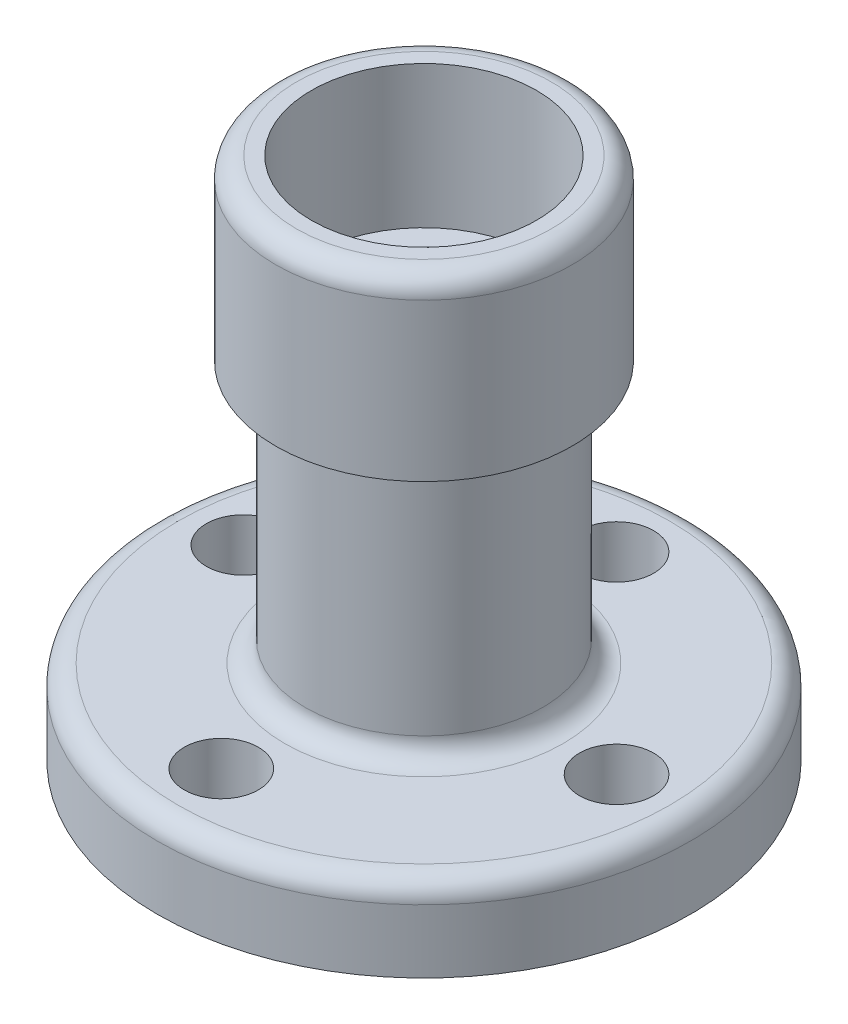
ISO-10303-21;
HEADER;
FILE_DESCRIPTION(('STEP AP214'),'2;1');
FILE_NAME('part.step','',(''),(''),'','','');
FILE_SCHEMA(('AUTOMOTIVE_DESIGN { 1 0 10303 214 1 1 1 1 }'));
ENDSEC;
DATA;
#1=APPLICATION_CONTEXT('core data for automotive mechanical design processes');
#2=APPLICATION_PROTOCOL_DEFINITION('international standard','automotive_design',2000,#1);
#3=PRODUCT_CONTEXT('',#1,'mechanical');
#4=PRODUCT('Part','Part','',(#3));
#5=PRODUCT_RELATED_PRODUCT_CATEGORY('part','',(#4));
#6=PRODUCT_DEFINITION_FORMATION('','',#4);
#7=PRODUCT_DEFINITION_CONTEXT('part definition',#1,'design');
#8=PRODUCT_DEFINITION('design','',#6,#7);
#9=PRODUCT_DEFINITION_SHAPE('','',#8);
#10=(LENGTH_UNIT() NAMED_UNIT(*) SI_UNIT(.MILLI.,.METRE.));
#11=(NAMED_UNIT(*) PLANE_ANGLE_UNIT() SI_UNIT($,.RADIAN.));
#12=(NAMED_UNIT(*) SI_UNIT($,.STERADIAN.) SOLID_ANGLE_UNIT());
#13=UNCERTAINTY_MEASURE_WITH_UNIT(LENGTH_MEASURE(1.E-05),#10,'distance_accuracy_value','');
#14=(GEOMETRIC_REPRESENTATION_CONTEXT(3) GLOBAL_UNCERTAINTY_ASSIGNED_CONTEXT((#13)) GLOBAL_UNIT_ASSIGNED_CONTEXT((#10,
#11,#12)) REPRESENTATION_CONTEXT('',''));
#15=CARTESIAN_POINT('',(0.,0.,0.));
#16=DIRECTION('',(0.,0.,1.));
#17=DIRECTION('',(1.,0.,0.));
#18=AXIS2_PLACEMENT_3D('',#15,#16,#17);
#19=CARTESIAN_POINT('',(0.,14.2,0.));
#20=DIRECTION('',(0.,-1.,0.));
#21=DIRECTION('',(0.,0.,-1.));
#22=AXIS2_PLACEMENT_3D('',#19,#20,#21);
#23=CYLINDRICAL_SURFACE('',#22,45.);
#24=CARTESIAN_POINT('',(0.,10.7,0.));
#25=DIRECTION('',(0.,1.,0.));
#26=DIRECTION('',(0.,0.,1.));
#27=AXIS2_PLACEMENT_3D('',#24,#25,#26);
#28=CIRCLE('',#27,45.);
#29=CARTESIAN_POINT('',(0.,10.7,45.));
#30=VERTEX_POINT('',#29);
#31=EDGE_CURVE('E10',#30,#30,#28,.F.);
#32=ORIENTED_EDGE('',*,*,#31,.T.);
#33=EDGE_LOOP('',(#32));
#34=FACE_BOUND('',#33,.T.);
#35=CARTESIAN_POINT('',(0.,0.,0.));
#36=DIRECTION('',(0.,1.,0.));
#37=DIRECTION('',(0.,0.,1.));
#38=AXIS2_PLACEMENT_3D('',#35,#36,#37);
#39=CIRCLE('',#38,45.);
#40=CARTESIAN_POINT('',(0.,0.,45.));
#41=VERTEX_POINT('',#40);
#42=EDGE_CURVE('E66',#41,#41,#39,.T.);
#43=ORIENTED_EDGE('',*,*,#42,.T.);
#44=EDGE_LOOP('',(#43));
#45=FACE_BOUND('',#44,.T.);
#46=ADVANCED_FACE('F40',(#34,#45),#23,.T.);
#47=CARTESIAN_POINT('',(0.,14.2,0.));
#48=DIRECTION('',(0.,1.,0.));
#49=DIRECTION('',(0.,0.,1.));
#50=AXIS2_PLACEMENT_3D('',#47,#48,#49);
#51=PLANE('',#50);
#52=CARTESIAN_POINT('',(0.,14.2,0.));
#53=DIRECTION('',(0.,1.,0.));
#54=DIRECTION('',(0.,0.,1.));
#55=AXIS2_PLACEMENT_3D('',#52,#53,#54);
#56=CIRCLE('',#55,41.5);
#57=CARTESIAN_POINT('',(0.,14.2,41.5));
#58=VERTEX_POINT('',#57);
#59=EDGE_CURVE('E42',#58,#58,#56,.T.);
#60=ORIENTED_EDGE('',*,*,#59,.T.);
#61=EDGE_LOOP('',(#60));
#62=FACE_BOUND('',#61,.T.);
#63=CARTESIAN_POINT('',(0.,14.2,0.));
#64=DIRECTION('',(0.,1.,0.));
#65=DIRECTION('',(0.,0.,1.));
#66=AXIS2_PLACEMENT_3D('',#63,#64,#65);
#67=CIRCLE('',#66,23.5);
#68=CARTESIAN_POINT('',(0.,14.2,23.5));
#69=VERTEX_POINT('',#68);
#70=EDGE_CURVE('E62',#69,#69,#67,.F.);
#71=ORIENTED_EDGE('',*,*,#70,.T.);
#72=EDGE_LOOP('',(#71));
#73=FACE_BOUND('',#72,.T.);
#74=CARTESIAN_POINT('',(-1.69244395993731,14.2,32.5));
#75=DIRECTION('',(0.,1.,0.));
#76=DIRECTION('',(0.,0.,1.));
#77=AXIS2_PLACEMENT_3D('',#74,#75,#76);
#78=CIRCLE('',#77,6.25);
#79=CARTESIAN_POINT('',(-1.69244395993731,14.2,38.75));
#80=VERTEX_POINT('',#79);
#81=EDGE_CURVE('E76',#80,#80,#78,.T.);
#82=ORIENTED_EDGE('',*,*,#81,.F.);
#83=EDGE_LOOP('',(#82));
#84=FACE_BOUND('',#83,.T.);
#85=CARTESIAN_POINT('',(-32.5,14.2,-2.03093275192457));
#86=DIRECTION('',(0.,1.,0.));
#87=DIRECTION('',(0.,0.,1.));
#88=AXIS2_PLACEMENT_3D('',#85,#86,#87);
#89=CIRCLE('',#88,6.25);
#90=CARTESIAN_POINT('',(-32.5,14.2,4.21906724807543));
#91=VERTEX_POINT('',#90);
#92=EDGE_CURVE('E80',#91,#91,#89,.T.);
#93=ORIENTED_EDGE('',*,*,#92,.F.);
#94=EDGE_LOOP('',(#93));
#95=FACE_BOUND('',#94,.T.);
#96=CARTESIAN_POINT('',(32.5,14.2,0.));
#97=DIRECTION('',(0.,1.,0.));
#98=DIRECTION('',(0.,0.,1.));
#99=AXIS2_PLACEMENT_3D('',#96,#97,#98);
#100=CIRCLE('',#99,6.25);
#101=CARTESIAN_POINT('',(32.5,14.2,6.25));
#102=VERTEX_POINT('',#101);
#103=EDGE_CURVE('E84',#102,#102,#100,.T.);
#104=ORIENTED_EDGE('',*,*,#103,.F.);
#105=EDGE_LOOP('',(#104));
#106=FACE_BOUND('',#105,.T.);
#107=CARTESIAN_POINT('',(0.,14.2,-32.5));
#108=DIRECTION('',(0.,1.,0.));
#109=DIRECTION('',(0.,0.,1.));
#110=AXIS2_PLACEMENT_3D('',#107,#108,#109);
#111=CIRCLE('',#110,6.25);
#112=CARTESIAN_POINT('',(0.,14.2,-26.25));
#113=VERTEX_POINT('',#112);
#114=EDGE_CURVE('E87',#113,#113,#111,.T.);
#115=ORIENTED_EDGE('',*,*,#114,.F.);
#116=EDGE_LOOP('',(#115));
#117=FACE_BOUND('',#116,.T.);
#118=ADVANCED_FACE('F121',(#62,#73,#84,#95,#106,#117),#51,.T.);
#119=CARTESIAN_POINT('',(0.,0.,0.));
#120=DIRECTION('',(0.,1.,0.));
#121=DIRECTION('',(0.,0.,1.));
#122=AXIS2_PLACEMENT_3D('',#119,#120,#121);
#123=PLANE('',#122);
#124=CARTESIAN_POINT('',(0.,0.,0.));
#125=DIRECTION('',(0.,-1.,0.));
#126=DIRECTION('',(0.,0.,-1.));
#127=AXIS2_PLACEMENT_3D('',#124,#125,#126);
#128=CIRCLE('',#127,15.);
#129=CARTESIAN_POINT('',(0.,0.,-15.));
#130=VERTEX_POINT('',#129);
#131=EDGE_CURVE('E73',#130,#130,#128,.T.);
#132=ORIENTED_EDGE('',*,*,#131,.F.);
#133=EDGE_LOOP('',(#132));
#134=FACE_BOUND('',#133,.T.);
#135=CARTESIAN_POINT('',(-1.69244395993731,0.,32.5));
#136=DIRECTION('',(0.,1.,0.));
#137=DIRECTION('',(0.,0.,1.));
#138=AXIS2_PLACEMENT_3D('',#135,#136,#137);
#139=CIRCLE('',#138,6.25);
#140=CARTESIAN_POINT('',(-1.69244395993731,0.,38.75));
#141=VERTEX_POINT('',#140);
#142=EDGE_CURVE('E74',#141,#141,#139,.T.);
#143=ORIENTED_EDGE('',*,*,#142,.T.);
#144=EDGE_LOOP('',(#143));
#145=FACE_BOUND('',#144,.T.);
#146=CARTESIAN_POINT('',(-32.5,0.,-2.03093275192457));
#147=DIRECTION('',(0.,1.,0.));
#148=DIRECTION('',(0.,0.,1.));
#149=AXIS2_PLACEMENT_3D('',#146,#147,#148);
#150=CIRCLE('',#149,6.25);
#151=CARTESIAN_POINT('',(-32.5,0.,4.21906724807543));
#152=VERTEX_POINT('',#151);
#153=EDGE_CURVE('E79',#152,#152,#150,.T.);
#154=ORIENTED_EDGE('',*,*,#153,.T.);
#155=EDGE_LOOP('',(#154));
#156=FACE_BOUND('',#155,.T.);
#157=CARTESIAN_POINT('',(32.5,0.,0.));
#158=DIRECTION('',(0.,1.,0.));
#159=DIRECTION('',(0.,0.,1.));
#160=AXIS2_PLACEMENT_3D('',#157,#158,#159);
#161=CIRCLE('',#160,6.25);
#162=CARTESIAN_POINT('',(32.5,0.,6.25));
#163=VERTEX_POINT('',#162);
#164=EDGE_CURVE('E82',#163,#163,#161,.T.);
#165=ORIENTED_EDGE('',*,*,#164,.T.);
#166=EDGE_LOOP('',(#165));
#167=FACE_BOUND('',#166,.T.);
#168=CARTESIAN_POINT('',(0.,0.,-32.5));
#169=DIRECTION('',(0.,1.,0.));
#170=DIRECTION('',(0.,0.,1.));
#171=AXIS2_PLACEMENT_3D('',#168,#169,#170);
#172=CIRCLE('',#171,6.25);
#173=CARTESIAN_POINT('',(0.,0.,-26.25));
#174=VERTEX_POINT('',#173);
#175=EDGE_CURVE('E90',#174,#174,#172,.T.);
#176=ORIENTED_EDGE('',*,*,#175,.T.);
#177=EDGE_LOOP('',(#176));
#178=FACE_BOUND('',#177,.T.);
#179=ORIENTED_EDGE('',*,*,#42,.F.);
#180=EDGE_LOOP('',(#179));
#181=FACE_BOUND('',#180,.T.);
#182=ADVANCED_FACE('F119',(#134,#145,#156,#167,#178,#181),#123,.F.);
#183=CARTESIAN_POINT('',(0.,58.4,0.));
#184=DIRECTION('',(0.,-1.,0.));
#185=DIRECTION('',(0.,0.,-1.));
#186=AXIS2_PLACEMENT_3D('',#183,#184,#185);
#187=CYLINDRICAL_SURFACE('',#186,20.);
#188=CARTESIAN_POINT('',(0.,54.9,0.));
#189=DIRECTION('',(0.,1.,0.));
#190=DIRECTION('',(0.,0.,1.));
#191=AXIS2_PLACEMENT_3D('',#188,#189,#190);
#192=CIRCLE('',#191,20.);
#193=CARTESIAN_POINT('',(0.,54.9,20.));
#194=VERTEX_POINT('',#193);
#195=EDGE_CURVE('E48',#194,#194,#192,.F.);
#196=ORIENTED_EDGE('',*,*,#195,.T.);
#197=EDGE_LOOP('',(#196));
#198=FACE_BOUND('',#197,.T.);
#199=CARTESIAN_POINT('',(0.,17.7,0.));
#200=DIRECTION('',(0.,1.,0.));
#201=DIRECTION('',(0.,0.,1.));
#202=AXIS2_PLACEMENT_3D('',#199,#200,#201);
#203=CIRCLE('',#202,20.);
#204=CARTESIAN_POINT('',(0.,17.7,20.));
#205=VERTEX_POINT('',#204);
#206=EDGE_CURVE('E67',#205,#205,#203,.T.);
#207=ORIENTED_EDGE('',*,*,#206,.T.);
#208=EDGE_LOOP('',(#207));
#209=FACE_BOUND('',#208,.T.);
#210=ADVANCED_FACE('F124',(#198,#209),#187,.T.);
#211=CARTESIAN_POINT('',(0.,88.4,0.));
#212=DIRECTION('',(0.,-1.,0.));
#213=DIRECTION('',(0.,0.,-1.));
#214=AXIS2_PLACEMENT_3D('',#211,#212,#213);
#215=CYLINDRICAL_SURFACE('',#214,25.);
#216=CARTESIAN_POINT('',(0.,84.9,0.));
#217=DIRECTION('',(0.,1.,0.));
#218=DIRECTION('',(0.,0.,1.));
#219=AXIS2_PLACEMENT_3D('',#216,#217,#218);
#220=CIRCLE('',#219,25.);
#221=CARTESIAN_POINT('',(0.,84.9,25.));
#222=VERTEX_POINT('',#221);
#223=EDGE_CURVE('E60',#222,#222,#220,.F.);
#224=ORIENTED_EDGE('',*,*,#223,.T.);
#225=EDGE_LOOP('',(#224));
#226=FACE_BOUND('',#225,.T.);
#227=CARTESIAN_POINT('',(0.,58.4,0.));
#228=DIRECTION('',(0.,1.,0.));
#229=DIRECTION('',(0.,0.,1.));
#230=AXIS2_PLACEMENT_3D('',#227,#228,#229);
#231=CIRCLE('',#230,25.);
#232=CARTESIAN_POINT('',(0.,58.4,25.));
#233=VERTEX_POINT('',#232);
#234=EDGE_CURVE('E88',#233,#233,#231,.T.);
#235=ORIENTED_EDGE('',*,*,#234,.T.);
#236=EDGE_LOOP('',(#235));
#237=FACE_BOUND('',#236,.T.);
#238=ADVANCED_FACE('F167',(#226,#237),#215,.T.);
#239=CARTESIAN_POINT('',(0.,88.4,0.));
#240=DIRECTION('',(0.,1.,0.));
#241=DIRECTION('',(0.,0.,1.));
#242=AXIS2_PLACEMENT_3D('',#239,#240,#241);
#243=PLANE('',#242);
#244=CARTESIAN_POINT('',(0.,88.4,0.));
#245=DIRECTION('',(0.,1.,0.));
#246=DIRECTION('',(0.,0.,1.));
#247=AXIS2_PLACEMENT_3D('',#244,#245,#246);
#248=CIRCLE('',#247,21.5);
#249=CARTESIAN_POINT('',(0.,88.4,21.5));
#250=VERTEX_POINT('',#249);
#251=EDGE_CURVE('E58',#250,#250,#248,.T.);
#252=ORIENTED_EDGE('',*,*,#251,.T.);
#253=EDGE_LOOP('',(#252));
#254=FACE_BOUND('',#253,.T.);
#255=CARTESIAN_POINT('',(0.,88.4,0.));
#256=DIRECTION('',(0.,1.,0.));
#257=DIRECTION('',(0.,0.,1.));
#258=AXIS2_PLACEMENT_3D('',#255,#256,#257);
#259=CIRCLE('',#258,19.);
#260=CARTESIAN_POINT('',(0.,88.4,19.));
#261=VERTEX_POINT('',#260);
#262=EDGE_CURVE('E101',#261,#261,#259,.T.);
#263=ORIENTED_EDGE('',*,*,#262,.F.);
#264=EDGE_LOOP('',(#263));
#265=FACE_BOUND('',#264,.T.);
#266=ADVANCED_FACE('F168',(#254,#265),#243,.T.);
#267=CARTESIAN_POINT('',(0.,58.4,0.));
#268=DIRECTION('',(0.,1.,0.));
#269=DIRECTION('',(0.,0.,1.));
#270=AXIS2_PLACEMENT_3D('',#267,#268,#269);
#271=PLANE('',#270);
#272=CARTESIAN_POINT('',(0.,58.4,0.));
#273=DIRECTION('',(0.,1.,0.));
#274=DIRECTION('',(0.,0.,1.));
#275=AXIS2_PLACEMENT_3D('',#272,#273,#274);
#276=CIRCLE('',#275,23.5);
#277=CARTESIAN_POINT('',(0.,58.4,23.5));
#278=VERTEX_POINT('',#277);
#279=EDGE_CURVE('E55',#278,#278,#276,.T.);
#280=ORIENTED_EDGE('',*,*,#279,.T.);
#281=EDGE_LOOP('',(#280));
#282=FACE_BOUND('',#281,.T.);
#283=ORIENTED_EDGE('',*,*,#234,.F.);
#284=EDGE_LOOP('',(#283));
#285=FACE_BOUND('',#284,.T.);
#286=ADVANCED_FACE('F161',(#282,#285),#271,.F.);
#287=CARTESIAN_POINT('',(0.,-15.8,-32.5));
#288=DIRECTION('',(0.,1.,0.));
#289=DIRECTION('',(0.,0.,1.));
#290=AXIS2_PLACEMENT_3D('',#287,#288,#289);
#291=CYLINDRICAL_SURFACE('',#290,6.25);
#292=ORIENTED_EDGE('',*,*,#114,.T.);
#293=EDGE_LOOP('',(#292));
#294=FACE_BOUND('',#293,.T.);
#295=ORIENTED_EDGE('',*,*,#175,.F.);
#296=EDGE_LOOP('',(#295));
#297=FACE_BOUND('',#296,.T.);
#298=ADVANCED_FACE('F164',(#294,#297),#291,.F.);
#299=CARTESIAN_POINT('',(32.5,-15.8,0.));
#300=DIRECTION('',(0.,1.,0.));
#301=DIRECTION('',(0.,0.,1.));
#302=AXIS2_PLACEMENT_3D('',#299,#300,#301);
#303=CYLINDRICAL_SURFACE('',#302,6.25);
#304=ORIENTED_EDGE('',*,*,#103,.T.);
#305=EDGE_LOOP('',(#304));
#306=FACE_BOUND('',#305,.T.);
#307=ORIENTED_EDGE('',*,*,#164,.F.);
#308=EDGE_LOOP('',(#307));
#309=FACE_BOUND('',#308,.T.);
#310=ADVANCED_FACE('F184',(#306,#309),#303,.F.);
#311=CARTESIAN_POINT('',(-32.5,-15.8,-2.03093275192457));
#312=DIRECTION('',(0.,1.,0.));
#313=DIRECTION('',(0.,0.,1.));
#314=AXIS2_PLACEMENT_3D('',#311,#312,#313);
#315=CYLINDRICAL_SURFACE('',#314,6.25);
#316=ORIENTED_EDGE('',*,*,#92,.T.);
#317=EDGE_LOOP('',(#316));
#318=FACE_BOUND('',#317,.T.);
#319=ORIENTED_EDGE('',*,*,#153,.F.);
#320=EDGE_LOOP('',(#319));
#321=FACE_BOUND('',#320,.T.);
#322=ADVANCED_FACE('F186',(#318,#321),#315,.F.);
#323=CARTESIAN_POINT('',(-1.69244395993731,-15.8,32.5));
#324=DIRECTION('',(0.,1.,0.));
#325=DIRECTION('',(0.,0.,1.));
#326=AXIS2_PLACEMENT_3D('',#323,#324,#325);
#327=CYLINDRICAL_SURFACE('',#326,6.25);
#328=ORIENTED_EDGE('',*,*,#81,.T.);
#329=EDGE_LOOP('',(#328));
#330=FACE_BOUND('',#329,.T.);
#331=ORIENTED_EDGE('',*,*,#142,.F.);
#332=EDGE_LOOP('',(#331));
#333=FACE_BOUND('',#332,.T.);
#334=ADVANCED_FACE('F192',(#330,#333),#327,.F.);
#335=CARTESIAN_POINT('',(0.,76.4,0.));
#336=DIRECTION('',(0.,1.,0.));
#337=DIRECTION('',(0.,0.,1.));
#338=AXIS2_PLACEMENT_3D('',#335,#336,#337);
#339=CYLINDRICAL_SURFACE('',#338,19.);
#340=ORIENTED_EDGE('',*,*,#262,.T.);
#341=EDGE_LOOP('',(#340));
#342=FACE_BOUND('',#341,.T.);
#343=CARTESIAN_POINT('',(0.,64.4,0.));
#344=DIRECTION('',(0.,1.,0.));
#345=DIRECTION('',(0.,0.,1.));
#346=AXIS2_PLACEMENT_3D('',#343,#344,#345);
#347=CIRCLE('',#346,19.);
#348=CARTESIAN_POINT('',(0.,64.4,19.));
#349=VERTEX_POINT('',#348);
#350=EDGE_CURVE('E106',#349,#349,#347,.T.);
#351=ORIENTED_EDGE('',*,*,#350,.F.);
#352=EDGE_LOOP('',(#351));
#353=FACE_BOUND('',#352,.T.);
#354=ADVANCED_FACE('F200',(#342,#353),#339,.F.);
#355=CARTESIAN_POINT('',(0.,64.4,0.));
#356=DIRECTION('',(0.,1.,0.));
#357=DIRECTION('',(0.,0.,1.));
#358=AXIS2_PLACEMENT_3D('',#355,#356,#357);
#359=PLANE('',#358);
#360=CARTESIAN_POINT('',(0.,64.4,0.));
#361=DIRECTION('',(0.,1.,0.));
#362=DIRECTION('',(0.,0.,1.));
#363=AXIS2_PLACEMENT_3D('',#360,#361,#362);
#364=CIRCLE('',#363,15.);
#365=CARTESIAN_POINT('',(0.,64.4,15.));
#366=VERTEX_POINT('',#365);
#367=EDGE_CURVE('E107',#366,#366,#364,.T.);
#368=ORIENTED_EDGE('',*,*,#367,.F.);
#369=EDGE_LOOP('',(#368));
#370=FACE_BOUND('',#369,.T.);
#371=ORIENTED_EDGE('',*,*,#350,.T.);
#372=EDGE_LOOP('',(#371));
#373=FACE_BOUND('',#372,.T.);
#374=ADVANCED_FACE('F202',(#370,#373),#359,.T.);
#375=CARTESIAN_POINT('',(0.,58.4,0.));
#376=DIRECTION('',(0.,1.,0.));
#377=DIRECTION('',(0.,0.,1.));
#378=AXIS2_PLACEMENT_3D('',#375,#376,#377);
#379=CYLINDRICAL_SURFACE('',#378,15.);
#380=ORIENTED_EDGE('',*,*,#367,.T.);
#381=EDGE_LOOP('',(#380));
#382=FACE_BOUND('',#381,.T.);
#383=CARTESIAN_POINT('',(0.,3.5,0.));
#384=DIRECTION('',(0.,-1.,0.));
#385=DIRECTION('',(0.,0.,-1.));
#386=AXIS2_PLACEMENT_3D('',#383,#384,#385);
#387=CIRCLE('',#386,15.);
#388=CARTESIAN_POINT('',(0.,3.5,-15.));
#389=VERTEX_POINT('',#388);
#390=EDGE_CURVE('E68',#389,#389,#387,.T.);
#391=ORIENTED_EDGE('',*,*,#390,.T.);
#392=EDGE_LOOP('',(#391));
#393=FACE_BOUND('',#392,.T.);
#394=ADVANCED_FACE('F201',(#382,#393),#379,.F.);
#395=CARTESIAN_POINT('',(0.,0.,0.));
#396=DIRECTION('',(0.,1.,0.));
#397=DIRECTION('',(0.,0.,-1.));
#398=AXIS2_PLACEMENT_3D('',#395,#396,#397);
#399=CONICAL_SURFACE('',#398,15.,0.0610865238198017);
#400=CARTESIAN_POINT('',(0.,3.5,0.));
#401=DIRECTION('',(0.,-1.,0.));
#402=DIRECTION('',(0.,0.,-1.));
#403=AXIS2_PLACEMENT_3D('',#400,#401,#402);
#404=CIRCLE('',#403,15.2140691705267);
#405=CARTESIAN_POINT('',(0.,3.5,-15.2140691705267));
#406=VERTEX_POINT('',#405);
#407=EDGE_CURVE('E115',#406,#406,#404,.T.);
#408=ORIENTED_EDGE('',*,*,#407,.F.);
#409=EDGE_LOOP('',(#408));
#410=FACE_BOUND('',#409,.T.);
#411=ORIENTED_EDGE('',*,*,#131,.T.);
#412=EDGE_LOOP('',(#411));
#413=FACE_BOUND('',#412,.T.);
#414=ADVANCED_FACE('F117',(#410,#413),#399,.F.);
#415=CARTESIAN_POINT('',(0.,3.5,0.));
#416=DIRECTION('',(0.,-1.,0.));
#417=DIRECTION('',(0.,0.,-1.));
#418=AXIS2_PLACEMENT_3D('',#415,#416,#417);
#419=PLANE('',#418);
#420=ORIENTED_EDGE('',*,*,#390,.F.);
#421=EDGE_LOOP('',(#420));
#422=FACE_BOUND('',#421,.T.);
#423=ORIENTED_EDGE('',*,*,#407,.T.);
#424=EDGE_LOOP('',(#423));
#425=FACE_BOUND('',#424,.T.);
#426=ADVANCED_FACE('F147',(#422,#425),#419,.T.);
#427=CARTESIAN_POINT('',(0.,17.7,0.));
#428=DIRECTION('',(0.,1.,0.));
#429=DIRECTION('',(0.,0.,1.));
#430=AXIS2_PLACEMENT_3D('',#427,#428,#429);
#431=TOROIDAL_SURFACE('',#430,23.5,3.5);
#432=ORIENTED_EDGE('',*,*,#70,.F.);
#433=EDGE_LOOP('',(#432));
#434=FACE_BOUND('',#433,.T.);
#435=ORIENTED_EDGE('',*,*,#206,.F.);
#436=EDGE_LOOP('',(#435));
#437=FACE_BOUND('',#436,.T.);
#438=ADVANCED_FACE('F144',(#434,#437),#431,.F.);
#439=CARTESIAN_POINT('',(0.,84.9,0.));
#440=DIRECTION('',(0.,1.,0.));
#441=DIRECTION('',(0.,0.,1.));
#442=AXIS2_PLACEMENT_3D('',#439,#440,#441);
#443=TOROIDAL_SURFACE('',#442,21.5,3.5);
#444=ORIENTED_EDGE('',*,*,#223,.F.);
#445=EDGE_LOOP('',(#444));
#446=FACE_BOUND('',#445,.T.);
#447=ORIENTED_EDGE('',*,*,#251,.F.);
#448=EDGE_LOOP('',(#447));
#449=FACE_BOUND('',#448,.T.);
#450=ADVANCED_FACE('F149',(#446,#449),#443,.T.);
#451=CARTESIAN_POINT('',(0.,54.9,0.));
#452=DIRECTION('',(0.,1.,0.));
#453=DIRECTION('',(0.,0.,1.));
#454=AXIS2_PLACEMENT_3D('',#451,#452,#453);
#455=TOROIDAL_SURFACE('',#454,23.5,3.5);
#456=ORIENTED_EDGE('',*,*,#195,.F.);
#457=EDGE_LOOP('',(#456));
#458=FACE_BOUND('',#457,.T.);
#459=ORIENTED_EDGE('',*,*,#279,.F.);
#460=EDGE_LOOP('',(#459));
#461=FACE_BOUND('',#460,.T.);
#462=ADVANCED_FACE('F152',(#458,#461),#455,.F.);
#463=CARTESIAN_POINT('',(0.,10.7,0.));
#464=DIRECTION('',(0.,1.,0.));
#465=DIRECTION('',(0.,0.,1.));
#466=AXIS2_PLACEMENT_3D('',#463,#464,#465);
#467=TOROIDAL_SURFACE('',#466,41.5,3.5);
#468=ORIENTED_EDGE('',*,*,#31,.F.);
#469=EDGE_LOOP('',(#468));
#470=FACE_BOUND('',#469,.T.);
#471=ORIENTED_EDGE('',*,*,#59,.F.);
#472=EDGE_LOOP('',(#471));
#473=FACE_BOUND('',#472,.T.);
#474=ADVANCED_FACE('F39',(#470,#473),#467,.T.);
#475=CLOSED_SHELL('',(#46,#118,#182,#210,#238,#266,#286,#298,#310,#322,#334,#354,#374,#394,#414,
#426,#438,#450,#462,#474));
#476=MANIFOLD_SOLID_BREP('B2',#475);
#477=ADVANCED_BREP_SHAPE_REPRESENTATION('',(#18,#476),#14);
#478=SHAPE_DEFINITION_REPRESENTATION(#9,#477);
ENDSEC;
END-ISO-10303-21;
